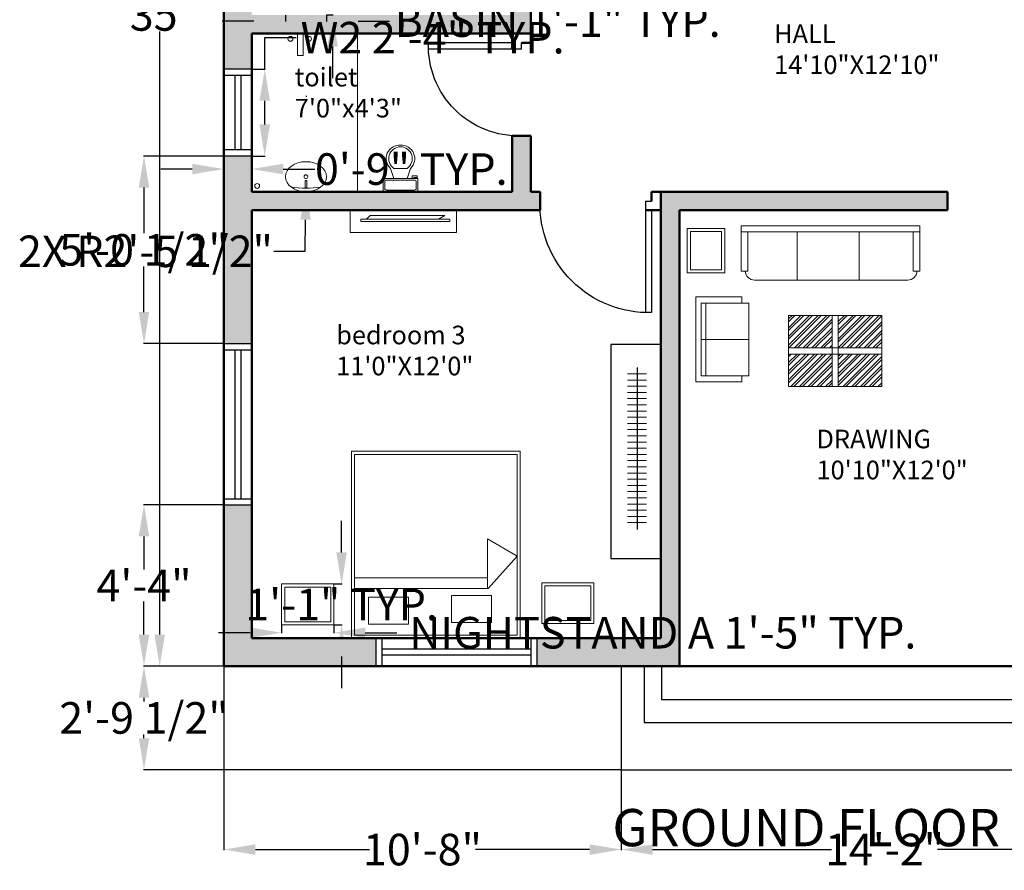
# Model space of a CAD drawing. Units: inches. Extents: x 18 to 9768, y 4 to 3529.
# Tile 1 of 6: x 8688 to 9006, y 3002 to 3276. Entities that reach past the tile are written whole.
import ezdxf

# ---------------------------------------------------------------- set-up
doc = ezdxf.new("R2010")
doc.units = ezdxf.units.IN
doc.header["$MEASUREMENT"] = 0
for name, color, linetype, lineweight in [('A-ANNO-DIMS', 2, 'Continuous', 18), ('A-ANNO-TEXT', 7, 'Continuous', 25), ('A-AREA-IDEN', 7, 'Continuous', 18), ('A-CASE-PATT', 9, 'Continuous', 13), ('A-EQPM', 8, 'Continuous', 18), ('A-FLOR-CASE', 9, 'Continuous', 25), ('A-FLOR-FIXT', 9, 'Continuous', 18), ('A-FLOR-STRS', 7, 'Continuous', 25), ('A-FURN', 8, 'Continuous', 18), ('A-FURN-PATT', 9, 'Continuous', 13), ('A-WALL-PATT', 252, 'Continuous', 13), ('WAL', 7, 'Continuous', 50)]:
    doc.layers.add(name, color=color, linetype=linetype, lineweight=lineweight)
doc.layers.add('A-DOOR', color=30, linetype='Continuous', lineweight=25, true_color=0xf8991e)
doc.layers.add('A-GLAZ', color=177, linetype='Continuous', lineweight=25, true_color=0x293189)
doc.styles.get("Standard").update_dxf_attribs({"font": 'arial.ttf'})
doc.dimstyles.get("Standard").update_dxf_attribs({"dimtxt": 10.18, "dimasz": 10.18, "dimexe": 0.18, "dimexo": 0.0625, "dimgap": 0.09, "dimtad": 0, "dimtih": 1, "dimtoh": 1, "dimdec": 0, "dimzin": 0, "dimdsep": 46, "dimlunit": 3, "dimtxsty": 'Standard', "dimcen": 0.09, "dimadec": 0, "dimazin": 0, "dimtfac": 1, "dimtdec": 0, "dimtofl": 0, "dimtmove": 0, "dimatfit": 3, "dimfxl": 1, "dimtolj": 1, "dimtzin": 0, "dimarcsym": 0})

# ---------------------------------------------------------------- blocks, each defined once
blk = doc.blocks.new('*U2')
for p, q in [((9.5, -6), (9.5, -2)), ((-10, -8.5), (-8, -8.5)), ((-10, -9.5), (-10, -8.5)), ((-7, -9.5), (-10, -9.5)), ((-8, -8.5), (-8, -8)), ((-7, -8), (-7, -9.5)), ((-4, -8), (-6, -14)), ((4, -8), (6, -14)), ((4, -14), (-4, -14))]:
    blk.add_line(p, q)
blk.add_lwpolyline([(10.5, -8), (10.5, 0), (-10.5, 0), (-10.5, -8)], close=True)
for points in [[(-9.5, -2), (-9.5, -6)], [(8.5, -1), (-8.5, -1)], [(-8.5, -7), (8.5, -7)]]:
    blk.add_lwpolyline(points)
for centre, radius, start, end in [((-8.625, -1.875), 0.8839, 81.8699, 188.1301), ((8.625, -1.875), 0.8839, 351.8699, 98.1301), ((-8.625, -6.125), 0.8839, 171.869898, 278.1301), ((8.625, -6.125), 0.8839, 261.8699, 8.1301), ((-0.4772, -19.9188), 8.0953, 133.01722, 273.38), ((0.0374, -19.8731), 7.127, 124.50543, 269.7), ((-0.0373, -19.8731), 7.127, 270.3, 55.4946), ((0.4773, -19.9188), 8.0953, 266.62, 46.9828)]:
    blk.add_arc(centre, radius, start, end)
blk = doc.blocks.new('*D4')
at = {"layer": 'A-ANNO-DIMS', "color": 0, "lineweight": -2, "transparency": 16777216}
for p, q in [((8753.82, 3487.73), (8733.02, 3487.73)), ((8733.2, 3477.55), (8733.2, 3283.03)), ((8733.2, 3077.91), (8733.2, 3272.44)), ((8753.82, 3067.73), (8733.02, 3067.73))]:
    blk.add_line(p, q, dxfattribs=at)
at = {"layer": 'A-ANNO-DIMS', "color": 0, "transparency": 16777216}
for points in [[(8731.5, 3477.55), (8734.9, 3477.55), (8733.2, 3487.73)], [(8731.5, 3077.91), (8734.9, 3077.91), (8733.2, 3067.73)]]:
    blk.add_solid(points, dxfattribs=at)
at = {"layer": 'Defpoints', "color": 0, "transparency": 16777216}
for p in [(8753.89, 3487.73), (8733.2, 3067.73), (8753.89, 3067.73)]:
    blk.add_point(p, dxfattribs=at)
at = {"layer": 'A-ANNO-DIMS', "color": 0, "transparency": 16777216, "insert": (8733.2, 3277.73), "char_height": 10.18, "attachment_point": 5}
blk.add_mtext("\\A1;35'", dxfattribs=at)
blk = doc.blocks.new('WINDOW-48')
for p, q in [((0, 0), (0, 9)), ((2, 0), (2, 9)), ((50, 0), (50, 9)), ((52, 0), (52, 9)), ((2, 5.5), (50, 5.5)), ((2, 3.5), (50, 3.5))]:
    blk.add_line(p, q)
blk = doc.blocks.new('WINDOW-24')
for p, q in [((9, 28), (0, 28)), ((9, 26), (0, 26)), ((3.5, 26), (3.5, 2)), ((5.5, 26), (5.5, 2)), ((9, 2), (0, 2)), ((9, 0), (0, 0))]:
    blk.add_line(p, q)
blk = doc.blocks.new('DOOR-36-W6')
for p, q in [((34.01, 0), (34.01, 36)), ((36.01, 3), (36.01, 36)), ((34.01, 0), (36.01, 0))]:
    blk.add_line(p, q)
blk.add_arc((35.01, 1), 35.01, 88.3634, 181.6366)
blk = doc.blocks.new('DOOR-30-W6')
for p, q in [((28.02, 30.02), (28.02, 0.02)), ((28.02, 30.02), (30.02, 30.02)), ((30.02, 27.02), (30.02, 0.02))]:
    blk.add_line(p, q)
blk.add_arc((29.02, 29.02), 29.02, 178.0251, 271.9749)
blk = doc.blocks.new('LAVATORY-OVAL')
for points in [[(6.91, 1.13), (6.91, 3.63), (6.32, 3.63), (6.32, 1.13)], [(6.32, 1.31), (6.32, 1.3), (6.91, 1.3), (6.91, 1.31)]]:
    blk.add_lwpolyline(points)
blk.add_circle((6.62, 4.84), 0.598)
blk.add_arc((6.8, 30.78), 29.65, 260.185, 278.8899)
blk.add_ellipse((6.62, 4.84), major_axis=(6.62, 0), ratio=0.731413)
blk = doc.blocks.new('NIGHTSTAND-RECT')
for points in [[(0, 13.21), (16.83, 13.21), (16.83, 0), (0, 0)], [(1, 12.21), (15.83, 12.21), (15.83, 1), (1, 1)]]:
    blk.add_lwpolyline(points, close=True)
blk = doc.blocks.new('*D27')
at = {"layer": 'A-ANNO-DIMS', "color": 0, "lineweight": -2, "transparency": 16777216}
for p, q in [((8767.09, 3260.23), (8767.09, 3270.41)), ((8767.09, 3270.41), (8777.27, 3270.41)), ((8762.95, 3260.23), (8767.27, 3260.23)), ((8767.09, 3242.41), (8767.09, 3250.05)), ((8762.95, 3232.23), (8767.27, 3232.23))]:
    blk.add_line(p, q, dxfattribs=at)
at = {"layer": 'A-ANNO-DIMS', "color": 0, "transparency": 16777216}
for points in [[(8765.39, 3250.05), (8768.78, 3250.05), (8767.09, 3260.23)], [(8765.39, 3242.41), (8768.78, 3242.41), (8767.09, 3232.23)]]:
    blk.add_solid(points, dxfattribs=at)
at = {"layer": 'Defpoints', "color": 0, "transparency": 16777216}
for p in [(8762.89, 3260.23), (8767.09, 3260.23), (8762.89, 3232.23)]:
    blk.add_point(p, dxfattribs=at)
at = {"layer": 'A-ANNO-DIMS', "color": 0, "transparency": 16777216, "insert": (8821.23, 3270.41), "char_height": 10.18, "attachment_point": 5}
blk.add_mtext('\\A1;W2 2\'-4" TYP.', dxfattribs=at)
blk = doc.blocks.new('*D28')
at = {"layer": 'A-ANNO-DIMS', "color": 0, "lineweight": -2, "transparency": 16777216}
for p, q in [((8753.89, 3232.17), (8753.89, 3227.85)), ((8762.89, 3232.17), (8762.89, 3227.85)), ((8743.71, 3228.03), (8733.53, 3228.03)), ((8773.07, 3228.03), (8783.25, 3228.03))]:
    blk.add_line(p, q, dxfattribs=at)
at = {"layer": 'A-ANNO-DIMS', "color": 0, "transparency": 16777216}
for points in [[(8743.71, 3229.73), (8743.71, 3226.34), (8753.89, 3228.03)], [(8773.07, 3229.73), (8773.07, 3226.34), (8762.89, 3228.03)]]:
    blk.add_solid(points, dxfattribs=at)
at = {"layer": 'Defpoints', "color": 0, "transparency": 16777216}
for p in [(8753.89, 3232.23), (8762.89, 3232.23), (8762.89, 3228.03)]:
    blk.add_point(p, dxfattribs=at)
at = {"layer": 'A-ANNO-DIMS', "color": 0, "transparency": 16777216, "insert": (8814.36, 3228.03), "char_height": 10.18, "attachment_point": 5}
blk.add_mtext('\\A1;0\'-9" TYP.', dxfattribs=at)
blk = doc.blocks.new('*D43')
at = {"layer": 'A-ANNO-DIMS', "color": 0, "lineweight": -2, "transparency": 16777216}
for p, q in [((8763.58, 3275.75), (8753.4, 3275.75)), ((8773.76, 3277.67), (8773.76, 3275.57)), ((8787, 3277.67), (8787, 3275.57)), ((8797.18, 3275.75), (8807.36, 3275.75))]:
    blk.add_line(p, q, dxfattribs=at)
at = {"layer": 'A-ANNO-DIMS', "color": 0, "transparency": 16777216}
for points in [[(8763.58, 3277.45), (8763.58, 3274.05), (8773.76, 3275.75)], [(8797.18, 3277.45), (8797.18, 3274.05), (8787, 3275.75)]]:
    blk.add_solid(points, dxfattribs=at)
at = {"layer": 'Defpoints', "color": 0, "transparency": 16777216}
for p in [(8773.76, 3277.73), (8787, 3277.73), (8787, 3275.75)]:
    blk.add_point(p, dxfattribs=at)
at = {"layer": 'A-ANNO-DIMS', "color": 0, "transparency": 16777216, "insert": (8861.56, 3275.75), "char_height": 10.18, "attachment_point": 5}
blk.add_mtext('\\A1;BASIN 1\'-1" TYP.', dxfattribs=at)
blk = doc.blocks.new('*D44')
at = {"layer": 'A-ANNO-DIMS', "color": 0, "lineweight": -2, "transparency": 16777216}
for p, q in [((8788.98, 3297.59), (8788.98, 3307.77)), ((8788.98, 3307.77), (8799.16, 3307.77)), ((8787.06, 3287.41), (8789.16, 3287.41)), ((8787.06, 3277.73), (8789.16, 3277.73)), ((8788.98, 3267.55), (8788.98, 3257.37))]:
    blk.add_line(p, q, dxfattribs=at)
at = {"layer": 'A-ANNO-DIMS', "color": 0, "transparency": 16777216}
for points in [[(8787.29, 3297.59), (8790.68, 3297.59), (8788.98, 3287.41)], [(8787.29, 3267.55), (8790.68, 3267.55), (8788.98, 3277.73)]]:
    blk.add_solid(points, dxfattribs=at)
at = {"layer": 'Defpoints', "color": 0, "transparency": 16777216}
for p in [(8787, 3287.41), (8788.98, 3287.41), (8787, 3277.73)]:
    blk.add_point(p, dxfattribs=at)
at = {"layer": 'A-ANNO-DIMS', "color": 0, "transparency": 16777216, "insert": (8842.14, 3307.77), "char_height": 10.18, "attachment_point": 5}
blk.add_mtext('\\A1;0\'-9 1/2" TYP.', dxfattribs=at)
blk = doc.blocks.new('*D53')
at = {"layer": 'A-ANNO-DIMS', "color": 0, "lineweight": -2, "transparency": 16777216}
for p, q in [((8772.54, 3080.95), (8772.54, 3078.31)), ((8789.36, 3080.95), (8789.36, 3078.31)), ((8762.36, 3078.49), (8752.18, 3078.49)), ((8799.54, 3078.49), (8809.72, 3078.49))]:
    blk.add_line(p, q, dxfattribs=at)
at = {"layer": 'A-ANNO-DIMS', "color": 0, "transparency": 16777216}
for points in [[(8762.36, 3080.19), (8762.36, 3076.79), (8772.54, 3078.49)], [(8799.54, 3080.19), (8799.54, 3076.79), (8789.36, 3078.49)]]:
    blk.add_solid(points, dxfattribs=at)
at = {"layer": 'Defpoints', "color": 0, "transparency": 16777216}
for p in [(8772.54, 3081.01), (8789.36, 3081.01), (8789.36, 3078.49)]:
    blk.add_point(p, dxfattribs=at)
at = {"layer": 'A-ANNO-DIMS', "color": 0, "transparency": 16777216, "insert": (8895.51, 3078.49), "char_height": 10.18, "attachment_point": 5}
blk.add_mtext('\\A1;NIGHTSTAND A 1\'-5" TYP.', dxfattribs=at)
blk = doc.blocks.new('*D54')
at = {"layer": 'A-ANNO-DIMS', "color": 0, "lineweight": -2, "transparency": 16777216}
for p, q in [((8791.89, 3104.4), (8791.89, 3114.58)), ((8789.43, 3094.22), (8792.07, 3094.22)), ((8789.43, 3081.01), (8792.07, 3081.01)), ((8791.89, 3070.83), (8791.89, 3060.65))]:
    blk.add_line(p, q, dxfattribs=at)
at = {"layer": 'A-ANNO-DIMS', "color": 0, "transparency": 16777216}
for points in [[(8790.19, 3104.4), (8793.58, 3104.4), (8791.89, 3094.22)], [(8790.19, 3070.83), (8793.58, 3070.83), (8791.89, 3081.01)]]:
    blk.add_solid(points, dxfattribs=at)
at = {"layer": 'Defpoints', "color": 0, "transparency": 16777216}
for p in [(8789.36, 3094.22), (8791.89, 3094.22), (8789.36, 3081.01)]:
    blk.add_point(p, dxfattribs=at)
at = {"layer": 'A-ANNO-DIMS', "color": 0, "transparency": 16777216, "insert": (8791.89, 3087.62), "char_height": 10.18, "attachment_point": 5}
blk.add_mtext('\\A1;1\'-1" TYP.', dxfattribs=at)
blk = doc.blocks.new('*D57')
at = {"layer": 'A-ANNO-DIMS', "color": 0, "lineweight": -2, "transparency": 16777216}
for p, q in [((8882.05, 3034.24), (8882.05, 3008.38)), ((9052.03, 3034.24), (9052.03, 3008.38)), ((8892.23, 3008.56), (8949.95, 3008.56)), ((9041.85, 3008.56), (8984.14, 3008.56))]:
    blk.add_line(p, q, dxfattribs=at)
at = {"layer": 'A-ANNO-DIMS', "color": 0, "transparency": 16777216}
for points in [[(8892.23, 3010.25), (8892.23, 3006.86), (8882.05, 3008.56)], [(9041.85, 3010.25), (9041.85, 3006.86), (9052.03, 3008.56)]]:
    blk.add_solid(points, dxfattribs=at)
at = {"layer": 'Defpoints', "color": 0, "transparency": 16777216}
for p in [(8882.05, 3034.31), (9052.03, 3034.31), (9052.03, 3008.56)]:
    blk.add_point(p, dxfattribs=at)
at = {"layer": 'A-ANNO-DIMS', "color": 0, "transparency": 16777216, "insert": (8967.04, 3008.56), "char_height": 10.18, "attachment_point": 5}
blk.add_mtext('\\A1;14\'-2"', dxfattribs=at)
blk = doc.blocks.new('*D58')
at = {"layer": 'A-ANNO-DIMS', "color": 0, "lineweight": -2, "transparency": 16777216}
for p, q in [((8881.99, 3067.73), (8727.96, 3067.73)), ((8728.14, 3057.55), (8728.14, 3056.37)), ((8728.14, 3044.49), (8728.14, 3045.67)), ((8881.99, 3034.31), (8727.96, 3034.31))]:
    blk.add_line(p, q, dxfattribs=at)
at = {"layer": 'A-ANNO-DIMS', "color": 0, "transparency": 16777216}
for points in [[(8726.44, 3057.55), (8729.83, 3057.55), (8728.14, 3067.73)], [(8726.44, 3044.49), (8729.83, 3044.49), (8728.14, 3034.31)]]:
    blk.add_solid(points, dxfattribs=at)
at = {"layer": 'Defpoints', "color": 0, "transparency": 16777216}
for p in [(8728.14, 3067.73), (8882.05, 3067.73), (8882.05, 3034.31)]:
    blk.add_point(p, dxfattribs=at)
at = {"layer": 'A-ANNO-DIMS', "color": 0, "transparency": 16777216, "insert": (8728.14, 3051.02), "char_height": 10.18, "attachment_point": 5}
blk.add_mtext('\\A1;2\'-9 1/2"', dxfattribs=at)
blk = doc.blocks.new('*D67')
at = {"layer": 'A-ANNO-DIMS', "color": 0, "lineweight": -2, "transparency": 16777216}
for p, q in [((8753.89, 3067.67), (8753.89, 3008.38)), ((8882.05, 3034.24), (8882.05, 3008.38)), ((8764.07, 3008.56), (8800.87, 3008.56)), ((8871.87, 3008.56), (8835.07, 3008.56))]:
    blk.add_line(p, q, dxfattribs=at)
at = {"layer": 'A-ANNO-DIMS', "color": 0, "transparency": 16777216}
for points in [[(8764.07, 3010.25), (8764.07, 3006.86), (8753.89, 3008.56)], [(8871.87, 3010.25), (8871.87, 3006.86), (8882.05, 3008.56)]]:
    blk.add_solid(points, dxfattribs=at)
at = {"layer": 'Defpoints', "color": 0, "transparency": 16777216}
for p in [(8753.89, 3067.73), (8882.05, 3034.31), (8882.05, 3008.56)]:
    blk.add_point(p, dxfattribs=at)
at = {"layer": 'A-ANNO-DIMS', "color": 0, "transparency": 16777216, "insert": (8817.97, 3008.56), "char_height": 10.18, "attachment_point": 5}
blk.add_mtext('\\A1;10\'-8"', dxfattribs=at)
blk = doc.blocks.new('*D75')
at = {"layer": 'A-ANNO-DIMS', "color": 0, "lineweight": -2, "transparency": 16777216}
for p, q in [((8753.82, 3119.73), (8727.96, 3119.73)), ((8728.14, 3109.55), (8728.14, 3098.91)), ((8728.14, 3077.91), (8728.14, 3088.55)), ((8753.82, 3067.73), (8727.96, 3067.73))]:
    blk.add_line(p, q, dxfattribs=at)
at = {"layer": 'A-ANNO-DIMS', "color": 0, "transparency": 16777216}
for points in [[(8726.44, 3109.55), (8729.83, 3109.55), (8728.14, 3119.73)], [(8726.44, 3077.91), (8729.83, 3077.91), (8728.14, 3067.73)]]:
    blk.add_solid(points, dxfattribs=at)
at = {"layer": 'Defpoints', "color": 0, "transparency": 16777216}
for p in [(8728.14, 3119.73), (8753.89, 3119.73), (8753.89, 3067.73)]:
    blk.add_point(p, dxfattribs=at)
at = {"layer": 'A-ANNO-DIMS', "color": 0, "transparency": 16777216, "insert": (8728.14, 3093.73), "char_height": 10.18, "attachment_point": 5}
blk.add_mtext('\\A1;4\'-4"', dxfattribs=at)
blk = doc.blocks.new('*D76')
at = {"layer": 'A-ANNO-DIMS', "color": 0, "lineweight": -2, "transparency": 16777216}
for p, q in [((8753.82, 3232.23), (8727.96, 3232.23)), ((8728.14, 3222.05), (8728.14, 3207.34)), ((8728.14, 3181.91), (8728.14, 3196.63)), ((8753.82, 3171.73), (8727.96, 3171.73))]:
    blk.add_line(p, q, dxfattribs=at)
at = {"layer": 'A-ANNO-DIMS', "color": 0, "transparency": 16777216}
for points in [[(8726.44, 3222.05), (8729.83, 3222.05), (8728.14, 3232.23)], [(8726.44, 3181.91), (8729.83, 3181.91), (8728.14, 3171.73)]]:
    blk.add_solid(points, dxfattribs=at)
at = {"layer": 'Defpoints', "color": 0, "transparency": 16777216}
for p in [(8728.14, 3232.23), (8753.89, 3232.23), (8753.89, 3171.73)]:
    blk.add_point(p, dxfattribs=at)
at = {"layer": 'A-ANNO-DIMS', "color": 0, "transparency": 16777216, "insert": (8728.14, 3201.98), "char_height": 10.18, "attachment_point": 5}
blk.add_mtext('\\A1;5\'-0 1/2"', dxfattribs=at)
blk = doc.blocks.new('*D85')
at = {"layer": 'A-ANNO-DIMS', "color": 0, "lineweight": -2, "transparency": 16777216}
for p, q in [((8780.48, 3251.52), (8780.66, 3251.52)), ((8780.57, 3251.43), (8780.57, 3251.61)), ((8780.16, 3201.5), (8780.25, 3211.68)), ((8769.98, 3201.5), (8780.16, 3201.5))]:
    blk.add_line(p, q, dxfattribs=at)
at = {"layer": 'A-ANNO-DIMS', "color": 0, "transparency": 16777216}
blk.add_solid([(8778.55, 3211.7), (8781.94, 3211.67), (8780.33, 3221.86)], dxfattribs=at)
at = {"layer": 'Defpoints', "color": 0, "transparency": 16777216}
for p in [(8780.57, 3251.52), (8780.33, 3221.86)]:
    blk.add_point(p, dxfattribs=at)
at = {"layer": 'A-ANNO-DIMS', "color": 0, "transparency": 16777216, "insert": (8728.61, 3201.5), "char_height": 10.18, "attachment_point": 5}
blk.add_mtext('\\A1;2X R2\'-5 1/2"', dxfattribs=at)

msp = doc.modelspace()

# ---------------------------------------------------------------- hatches: boundary and pattern name
at = {"layer": 'A-CASE-PATT'}
h = msp.add_hatch(dxfattribs=at)
h.set_pattern_fill('ANSI31', color=256, scale=16, angle=-45, style=0)
h.paths.add_polyline_path([(8884.1, 3112.17), (8890.21, 3112.17), (8890.21, 3162.17), (8884.1, 3162.17)])
at = {"layer": 'A-FURN-PATT'}
h = msp.add_hatch(dxfattribs=at)
h.set_pattern_fill('ANSI32', color=256, scale=5.3)
h.paths.add_polyline_path([(8966.14, 3180.79), (8952.12, 3180.79), (8952.12, 3170.34), (8966.14, 3170.34)])
h.paths.add_polyline_path([(8950.12, 3180.79), (8936.1, 3180.79), (8936.1, 3170.34), (8950.12, 3170.34)])
h.paths.add_polyline_path([(8950.12, 3168.34), (8936.1, 3168.34), (8936.1, 3157.89), (8950.12, 3157.89)])
h.paths.add_polyline_path([(8966.14, 3168.34), (8952.12, 3168.34), (8952.12, 3157.89), (8966.14, 3157.89)])
at = {"layer": 'A-WALL-PATT'}
h = msp.add_hatch(color=256, dxfattribs=at)
h.dxf.hatch_style = 1
h.paths.add_polyline_path([(8762.89, 3478.73), (8802.89, 3478.73), (8802.89, 3487.73), (8753.89, 3487.73), (8753.89, 3317.23), (8762.89, 3317.23), (8762.89, 3328.73), (8813.89, 3328.73), (8813.89, 3329.73, -0.017236), (8813.89, 3331.73), (8813.89, 3334.73), (8762.89, 3334.73)])
h.paths.add_polyline_path([(8900.89, 3487.73), (8854.89, 3487.73), (8854.89, 3478.73), (8894.89, 3478.73), (8894.89, 3421.46), (8894.89, 3334.73), (8894.89, 3328.73), (8900.89, 3328.73), (8900.89, 3391.73), (8900.89, 3478.73)])
h.paths.add_polyline_path([(9074.89, 3487.73), (9011.3, 3487.73), (9011.3, 3478.73), (9030.89, 3478.73), (9030.89, 3391.73), (8939.89, 3391.73), (8939.89, 3390.73, -0.014283), (8939.89, 3388.73), (8939.89, 3385.73), (9030.89, 3385.73), (9030.89, 3373.73), (9033.89, 3373.73, -0.014283), (9035.89, 3373.73), (9036.89, 3373.73), (9036.89, 3478.73), (9074.89, 3478.73)])
h.paths.add_polyline_path([(9173.89, 3487.73), (9126.89, 3487.73), (9126.89, 3478.73), (9128.34, 3478.73), (9164.89, 3478.73), (9164.89, 3334.73), (9147.51, 3334.73), (9036.89, 3334.73), (9030.89, 3334.73), (9030.89, 3328.73), (9164.89, 3328.73), (9164.89, 3300.73), (9173.89, 3300.73)])
h.paths.add_polyline_path([(8762.89, 3271.73), (8846.89, 3271.73), (8852.89, 3271.73), (8852.89, 3328.73), (8855.89, 3328.73), (8855.89, 3331.73, -0.014283), (8855.89, 3333.73), (8855.89, 3334.73), (8846.89, 3334.73), (8846.89, 3328.73), (8846.89, 3277.73), (8762.89, 3277.73), (8762.89, 3289.23), (8753.89, 3289.23), (8753.89, 3260.23), (8762.89, 3260.23)])
h.paths.add_polyline_path([(8762.89, 3214.73), (8855.89, 3214.73), (8855.89, 3215.73, -0.014283), (8855.89, 3217.73), (8855.89, 3220.73), (8852.89, 3220.73), (8852.89, 3238.73), (8849.89, 3238.73, -0.017236), (8847.89, 3238.73), (8846.89, 3238.73), (8846.89, 3220.73), (8762.89, 3220.73), (8762.89, 3232.23), (8753.89, 3232.23), (8753.89, 3171.73), (8762.89, 3171.73)])
h.paths.add_polyline_path([(8762.89, 3119.73), (8753.89, 3119.73), (8753.89, 3067.73), (8802.89, 3067.73), (8802.89, 3076.73), (8795.03, 3076.73), (8762.89, 3076.73)])
h.paths.add_polyline_path([(8900.89, 3076.73), (8900.89, 3214.73), (8987.37, 3214.73), (8987.37, 3220.73), (8894.89, 3220.73), (8894.89, 3214.73), (8894.89, 3076.73), (8854.89, 3076.73), (8854.89, 3067.73), (8900.89, 3067.73)])
h.paths.add_polyline_path([(9074.89, 3076.73), (9071.87, 3076.73), (9036.89, 3076.73), (9036.89, 3214.73), (9036.89, 3220.73), (9030.89, 3220.73), (9030.89, 3214.73), (9030.89, 3076.73), (9030.89, 3067.73), (9074.89, 3067.73)])
h.paths.add_polyline_path([(9173.89, 3119.73), (9164.89, 3119.73), (9164.89, 3076.73), (9126.89, 3076.73), (9126.89, 3067.73), (9173.89, 3067.73)])
h.paths.add_polyline_path([(9173.89, 3248.73), (9164.89, 3248.73), (9164.89, 3220.73), (9075.89, 3220.73), (9075.89, 3217.73, -0.014283), (9075.89, 3215.73), (9075.89, 3214.73), (9164.89, 3214.73), (9164.89, 3171.73), (9173.89, 3171.73)])

# ---------------------------------------------------------------- linework, layer by layer
at = {"layer": 'A-EQPM'}
for p, q in [((8799.95, 3211.84), (8801.05, 3213.07)), ((8801.05, 3213.07), (8825.15, 3213.07)), ((8825.15, 3213.07), (8823.18, 3211.84))]:
    msp.add_line(p, q, dxfattribs=at)
for points in [[(8794.7, 3214.73), (8828.93, 3214.73), (8828.93, 3207.61), (8794.7, 3207.61)], [(8798.05, 3211.84), (8826.77, 3211.84), (8826.77, 3211.09), (8798.05, 3211.09)]]:
    msp.add_lwpolyline(points, close=True, dxfattribs=at)
at = {"layer": 'A-FLOR-CASE'}
msp.add_line((8887.19, 3164.07), (8887.19, 3111.84), dxfattribs=at)
msp.add_lwpolyline([(8894.89, 3171.45), (8878.77, 3171.45), (8878.77, 3102.41), (8894.89, 3102.41)], close=True, dxfattribs=at)
at = {"layer": 'A-FLOR-FIXT'}
msp.add_line((8796.99, 3271.73), (8796.99, 3220.73), dxfattribs=at)
msp.add_lwpolyline([(8777.71, 3271.73), (8779.46, 3271.73), (8779.46, 3264.64), (8777.71, 3264.64)], close=True, dxfattribs=at)
for centre, radius in [((8775.39, 3270.03), 0.804), ((8781.37, 3270.03), 0.804), ((8764.63, 3222.59), 0.778)]:
    msp.add_circle(centre, radius, dxfattribs=at)
at = {"layer": 'A-FLOR-STRS'}
for p, q in [((8882.05, 3067.73), (8882.05, 3034.31)), ((8889.5, 3067.73), (8889.5, 3049.55)), ((8895.12, 3067.73), (8895.12, 3056.93)), ((8895.12, 3056.93), (9036.57, 3056.93)), ((8889.5, 3049.55), (9045.05, 3049.55)), ((8882.05, 3034.31), (9052.03, 3034.31))]:
    msp.add_line(p, q, dxfattribs=at)
at = {"layer": 'A-FURN'}
for p, q in [((8938.86, 3207.76), (8938.86, 3192.2)), ((8958.86, 3207.76), (8958.86, 3192.2)), ((8909.43, 3184.82), (8909.43, 3161.33)), ((8950.12, 3180.79), (8950.12, 3157.89)), ((8952.12, 3180.79), (8952.12, 3157.89)), ((8907.87, 3173.07), (8923.29, 3173.07)), ((8936.1, 3170.34), (8966.14, 3170.34)), ((8936.1, 3168.34), (8966.14, 3168.34)), ((8848.52, 3103.22), (8838.9, 3108.78)), ((8838.9, 3108.78), (8838.9, 3093.18)), ((8839.16, 3092.74), (8848.52, 3103.22)), ((8838.9, 3096.16), (8796.03, 3096.16)), ((8796.03, 3092.74), (8839.16, 3092.74)), ((8838.9, 3093.18), (8838.9, 3092.74))]:
    msp.add_line(p, q, dxfattribs=at)
for points in [[(8903.39, 3208.89), (8903.39, 3208.89), (8915.46, 3208.89), (8915.46, 3208.89), (8915.46, 3194.56), (8915.46, 3194.56), (8903.39, 3194.56), (8903.39, 3194.56)], [(8920.82, 3207.76), (8920.82, 3207.76), (8978.45, 3207.76), (8978.45, 3207.76), (8978.45, 3209.76), (8978.45, 3209.76), (8920.82, 3209.76), (8920.82, 3209.76)], [(8904.39, 3207.89), (8914.46, 3207.89), (8914.46, 3195.56), (8904.39, 3195.56)], [(8922.98, 3207.76), (8922.98, 3207.76), (8920.82, 3207.76), (8920.82, 3207.76), (8920.82, 3195.11), (8920.82, 3195.11), (8922.98, 3195.11), (8922.98, 3195.11)], [(8978.43, 3207.76), (8978.43, 3207.76), (8976.26, 3207.76), (8976.26, 3207.76), (8976.26, 3195.11), (8976.26, 3195.11), (8978.43, 3195.11), (8978.43, 3195.11)], [(8907.87, 3184.82), (8907.87, 3184.82), (8923.29, 3184.82), (8923.29, 3184.82), (8923.29, 3161.33), (8923.29, 3161.33), (8907.87, 3161.33), (8907.87, 3161.33)], [(8936.1, 3180.79), (8936.1, 3180.79), (8966.14, 3180.79), (8966.14, 3180.79), (8966.14, 3157.89), (8966.14, 3157.89), (8936.1, 3157.89), (8936.1, 3157.89)], [(8795.03, 3076.73), (8849.52, 3076.73), (8849.52, 3137), (8795.03, 3137)], [(8796.03, 3077.73), (8848.52, 3077.73), (8848.52, 3136), (8796.03, 3136)], [(8827.3, 3090.49), (8840.22, 3090.49), (8840.22, 3081.79), (8827.3, 3081.79)], [(8800.59, 3090), (8813.51, 3090), (8813.51, 3081.3), (8800.59, 3081.3)]]:
    msp.add_lwpolyline(points, close=True, dxfattribs=at)
msp.add_lwpolyline([(8977.5, 3195.11, -0.404999), (8974.5, 3192.2), (8925.1, 3192.2, -0.404999), (8922.1, 3195.11, -0.404999)], format="xyb", dxfattribs=at)
for points in [[(8907.87, 3184.82), (8920.95, 3184.82), (8920.95, 3184.82), (8920.95, 3186.8), (8920.95, 3186.8), (8906.16, 3186.8), (8906.16, 3186.8), (8906.16, 3184.82)], [(8906.16, 3184.82), (8906.16, 3184.82), (8906.16, 3161.33), (8906.16, 3161.33)], [(8907.87, 3161.33), (8907.87, 3161.33), (8907.87, 3184.82)], [(8906.16, 3161.34), (8906.16, 3161.34), (8906.16, 3159.36), (8906.16, 3159.36), (8920.95, 3159.36), (8920.95, 3159.36), (8920.95, 3161.34), (8920.95, 3161.34), (8907.87, 3161.34)]]:
    msp.add_lwpolyline(points, dxfattribs=at)
at = {"layer": 'WAL'}
for p, q in [((8753.89, 3067.73), (8753.89, 3487.73)), ((8852.89, 3271.73), (8852.89, 3328.73)), ((8762.89, 3271.73), (8846.89, 3271.73)), ((8762.89, 3220.73), (8762.89, 3271.73)), ((8846.89, 3271.73), (8852.89, 3271.73)), ((8846.89, 3266.73), (8846.89, 3271.73)), ((8852.89, 3268.73), (8852.89, 3271.73)), ((8849.89, 3268.73), (8852.89, 3268.73)), ((8846.89, 3220.73), (8846.89, 3238.79)), ((8846.89, 3238.73), (8852.89, 3238.73)), ((8852.89, 3220.73), (8852.89, 3238.73)), ((8762.89, 3220.73), (8846.89, 3220.73)), ((8846.89, 3220.73), (8762.89, 3220.73)), ((8852.89, 3220.73), (8855.89, 3220.73)), ((8855.89, 3220.73), (8852.89, 3220.73)), ((8855.89, 3214.73), (8855.89, 3220.73)), ((8891.89, 3217.73), (8891.89, 3220.73)), ((8891.89, 3220.73), (8900.89, 3220.73)), ((8987.37, 3220.73), (8891.89, 3220.73)), ((8894.89, 3214.73), (8894.89, 3220.73)), ((8987.37, 3220.73), (8987.37, 3214.73)), ((8762.89, 3076.73), (8762.89, 3214.73)), ((8762.89, 3214.73), (8855.93, 3214.73)), ((8855.93, 3214.73), (8762.89, 3214.73)), ((8894.89, 3214.73), (8889.89, 3214.73)), ((8889.89, 3214.73), (8894.89, 3214.73)), ((8894.89, 3076.73), (8894.89, 3214.73)), ((8900.89, 3076.73), (8900.89, 3214.73)), ((8987.37, 3214.73), (8900.89, 3214.73)), ((8894.89, 3076.73), (8762.89, 3076.73)), ((8900.89, 3076.73), (8900.89, 3067.73)), ((8900.89, 3067.73), (8753.89, 3067.73)), ((8900.89, 3067.73), (9030.89, 3067.73))]:
    msp.add_line(p, q, dxfattribs=at)

# ---------------------------------------------------------------- block references
at = {"layer": 'A-DOOR', "extrusion": (0, 0, -1), "zscale": -1}
for name, p, rotation in [('DOOR-30-W6', (-8819.87, 3238.72), 89.999999999982), ('DOOR-36-W6', (-8855.87, 3217.73), 180)]:
    msp.add_blockref(name, p, dxfattribs=dict(at, rotation=rotation))
at = {"layer": 'A-FLOR-FIXT', "xscale": 0.5359950384494228, "yscale": 0.5359950384494228, "zscale": 0.5359950384494228, "rotation": 180}
msp.add_blockref('*U2', (8810.88, 3220.73), dxfattribs=at)
at = {"layer": 'A-FLOR-FIXT'}
msp.add_blockref('LAVATORY-OVAL', (8773.76, 3220.73), dxfattribs=at)
at = {"layer": 'A-FURN'}
for p in [(8772.54, 3081.01), (8856.47, 3081.43)]:
    msp.add_blockref('NIGHTSTAND-RECT', p, dxfattribs=at)
at = {"layer": 'A-GLAZ'}
msp.add_blockref('WINDOW-24', (8753.89, 3232.24), dxfattribs=at)
for p, rotation in [((8753.89, 3171.73), 269.9999999999995), ((8854.89, 3076.73), 180)]:
    msp.add_blockref('WINDOW-48', p, dxfattribs=dict(at, rotation=rotation))

# ---------------------------------------------------------------- texts
at = {"layer": 'A-ANNO-TEXT', "insert": (8879.25, 3021.64), "char_height": 12, "attachment_point": 1}
msp.add_mtext_dynamic_manual_height_columns('GROUND FLOOR PLAN', width=342.8626, gutter_width=1, heights=[0], dxfattribs=at)
at = {"layer": 'A-AREA-IDEN', "char_height": 6, "attachment_point": 1}
for s, insert in [('HALL\\P14\'10"X12\'10"', (8931.41, 3274.67)), ('toilet\\P7\'0"x4\'3"', (8776.78, 3260.68)), ('bedroom 3\\P11\'0"X12\'0"', (8790.14, 3177.51)), ('DRAWING\\P10\'10"X12\'0"', (8945.07, 3143.98))]:
    msp.add_mtext_dynamic_manual_height_columns(s, width=53.4573, gutter_width=1, heights=[0], dxfattribs=dict(at, insert=insert))

# ---------------------------------------------------------------- dimensions: what is measured, and where the dimension line sits
at = {"layer": 'A-ANNO-DIMS'}
for base, p1, p2, override, picture, middle in [((8733.2, 3067.73), (8753.89, 3487.73), (8753.89, 3067.73), {"dimclrd": 0, "dimclre": 0, "dimclrt": 0}, '*D4', (8733.2, 3277.73)), ((8728.14, 3232.23), (8753.89, 3171.73), (8753.89, 3232.23), {"dimdec": 1, "dimlfac": 1, "dimrnd": 0, "dimzin": 1, "dimdsep": 46, "dimlunit": 4, "dimfrac": 2}, '*D76', (8728.14, 3201.98)), ((8728.14, 3119.73), (8753.89, 3067.73), (8753.89, 3119.73), {"dimdec": 1, "dimlfac": 1, "dimrnd": 0, "dimzin": 1, "dimdsep": 46, "dimlunit": 4, "dimfrac": 2}, '*D75', (8728.14, 3093.73)), ((8728.14, 3067.73), (8882.05, 3034.31), (8882.05, 3067.73), {"dimdec": 1, "dimlfac": 1, "dimrnd": 0, "dimzin": 1, "dimdsep": 46, "dimlunit": 4, "dimfrac": 2}, '*D58', (8728.14, 3051.02))]:
    dim = msp.add_linear_dim(base=base, p1=p1, p2=p2, angle=90, dimstyle='Standard', override=override, dxfattribs=at)
    dim.commit()
    dim.dimension.update_dxf_attribs({"geometry": picture, "text_midpoint": middle})
for base, p1, p2, text, picture, middle in [((8788.98, 3287.41), (8787, 3277.73), (8787, 3287.41), '<> TYP.', '*D44', (8842.14, 3307.77)), ((8767.09, 3260.23), (8762.89, 3232.23), (8762.89, 3260.23), 'W2 <> TYP.', '*D27', (8821.23, 3270.41)), ((8791.89, 3094.22), (8789.36, 3081.01), (8789.36, 3094.22), '<> TYP.', '*D54', (8791.89, 3087.62))]:
    dim = msp.add_linear_dim(base=base, p1=p1, p2=p2, angle=90, text=text, dimstyle='Standard', override={"dimdec": 1, "dimlfac": 1, "dimrnd": 0, "dimzin": 1, "dimdsep": 46, "dimlunit": 4, "dimfrac": 2}, dxfattribs=at)
    dim.commit()
    dim.dimension.update_dxf_attribs({"geometry": picture, "text_midpoint": middle})
for base, p1, p2, text, picture, middle in [((8787, 3275.75), (8773.76, 3277.73), (8787, 3277.73), 'BASIN <> TYP.', '*D43', (8861.56, 3275.75)), ((8762.89, 3228.03), (8753.89, 3232.23), (8762.89, 3232.23), '<> TYP.', '*D28', (8814.36, 3228.03)), ((8789.36, 3078.49), (8772.54, 3081.01), (8789.36, 3081.01), 'NIGHTSTAND A <> TYP.', '*D53', (8895.51, 3078.49))]:
    dim = msp.add_linear_dim(base=base, p1=p1, p2=p2, text=text, dimstyle='Standard', override={"dimdec": 1, "dimlfac": 1, "dimrnd": 0, "dimzin": 1, "dimdsep": 46, "dimlunit": 4, "dimfrac": 2}, dxfattribs=at)
    dim.commit()
    dim.dimension.update_dxf_attribs({"geometry": picture, "text_midpoint": middle})
dim = msp.add_radius_dim(center=(8780.57, 3251.52), mpoint=(8780.33, 3221.86), text='2X <>', dimstyle='Standard', override={"dimdec": 1, "dimlfac": 1, "dimrnd": 0, "dimzin": 1, "dimdsep": 46, "dimlunit": 4, "dimfrac": 2}, dxfattribs=at)
dim.commit()
dim.dimension.update_dxf_attribs({"geometry": '*D85', "text_midpoint": (8728.61, 3201.5)})
for base, p1, p2, picture, middle in [((8882.05, 3008.56), (8753.89, 3067.73), (8882.05, 3034.31), '*D67', (8817.97, 3008.56)), ((9052.03, 3008.56), (8882.05, 3034.31), (9052.03, 3034.31), '*D57', (8967.04, 3008.56))]:
    dim = msp.add_linear_dim(base=base, p1=p1, p2=p2, dimstyle='Standard', override={"dimdec": 1, "dimlfac": 1, "dimrnd": 0, "dimzin": 1, "dimdsep": 46, "dimlunit": 4, "dimfrac": 2}, dxfattribs=at)
    dim.commit()
    dim.dimension.update_dxf_attribs({"geometry": picture, "text_midpoint": middle})

doc.saveas('drawing.dxf')
